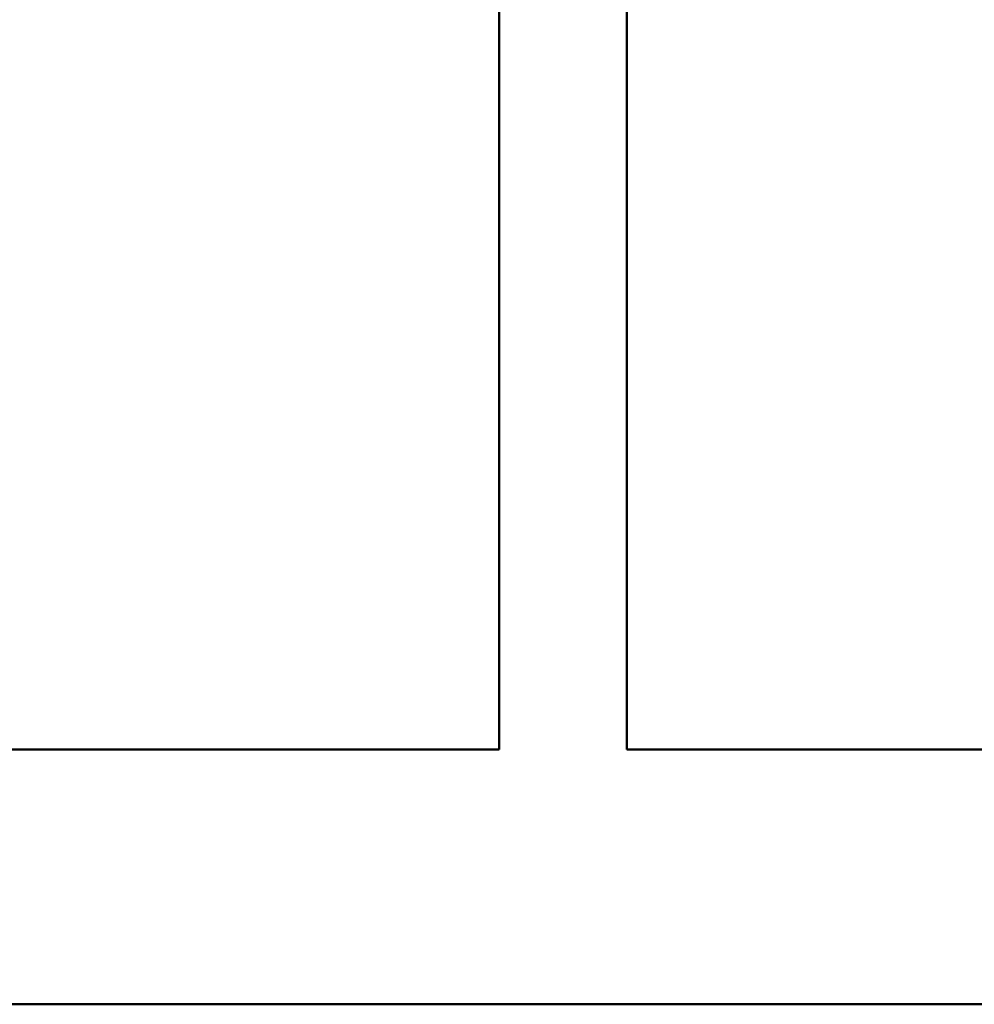
# Model space of a CAD drawing. Units: inches. Extents: x -173 to 545, y -746 to 104.
# Tile 12 of 32: x 339 to 373, y -697 to -663. Entities that reach past the tile are written whole.
import ezdxf

# ---------------------------------------------------------------- set-up
doc = ezdxf.new("R2010")
doc.units = ezdxf.units.IN
doc.header["$MEASUREMENT"] = 0
doc.layers.add('A-WALL', color=7, linetype='Continuous', lineweight=50)

msp = doc.modelspace()

# ---------------------------------------------------------------- linework, layer by layer
at = {"layer": 'A-WALL'}
for p, q in [((356.301, -551.862), (356.301, -688.362)), ((360.801, -551.862), (360.801, -688.362)), ((265.301, -688.362), (356.301, -688.362)), ((360.801, -688.362), (492.801, -688.362)), ((24.301, -697.362), (501.801, -697.362))]:
    msp.add_line(p, q, dxfattribs=at)

doc.saveas('drawing.dxf')
